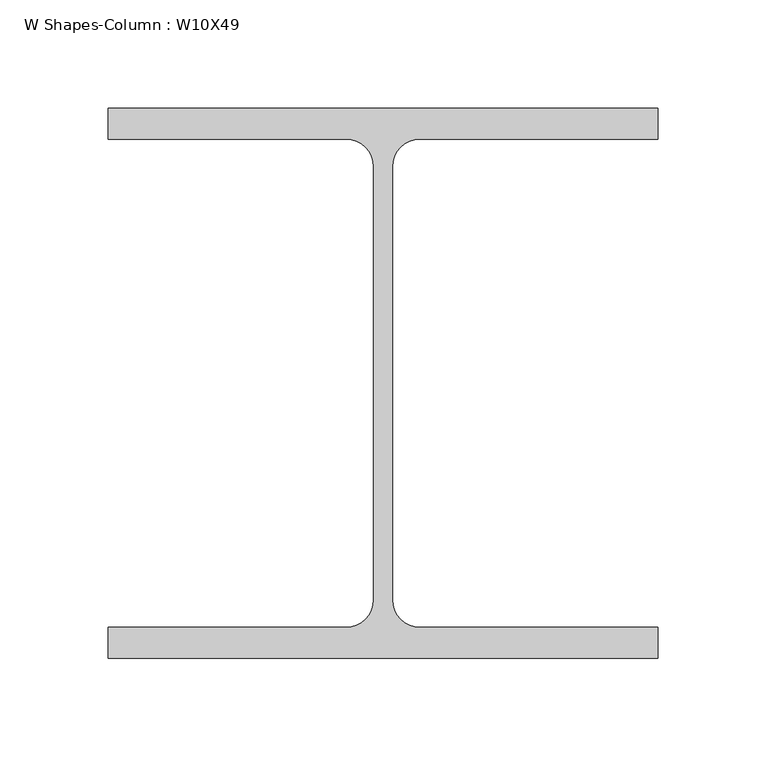
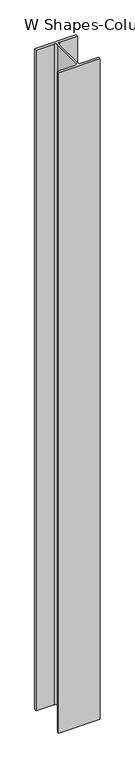
"""IFC4 building model written with IfcOpenShell, lengths in millimetres: column geometry, W Shapes-Column : W10X49."""

from ifc_helpers import new_model, si_unit, point, frame_2d, origin, origin_with_axes, place, context, project, spatial, polyline, circle_curve, trimmed, segment, composite_curve, outline, extrude, source, transform, mapped, element, save


def w_shapes_column_w10x49_053c6d64(model_context):
    return source(origin(), model_context, "Body", "SweptSolid", [
        extrude(outline(composite_curve([segment(polyline([(127.0, 127.0), (127.0, 112.776), (17.018, 112.776)]), True, "CONTINUOUS"), segment(trimmed(circle_curve(frame_2d((17.018, 100.076)), 12.7), [point((17.018, 112.776))], [point((4.318, 100.076))], True, "CARTESIAN"), True, "CONTINUOUS"), segment(polyline([(4.318, 100.076), (4.318, -100.076)]), True, "CONTINUOUS"), segment(trimmed(circle_curve(frame_2d((17.018, -100.076)), 12.7), [point((4.318, -100.076))], [point((17.018, -112.776))], True, "CARTESIAN"), True, "CONTINUOUS"), segment(polyline([(17.018, -112.776), (127.0, -112.776), (127.0, -127.0), (-127.0, -127.0), (-127.0, -112.776), (-17.018, -112.776)]), True, "CONTINUOUS"), segment(trimmed(circle_curve(frame_2d((-17.018, -100.076)), 12.7), [point((-17.018, -112.776))], [point((-4.318, -100.076))], True, "CARTESIAN"), True, "CONTINUOUS"), segment(polyline([(-4.318, -100.076), (-4.318, 100.076)]), True, "CONTINUOUS"), segment(trimmed(circle_curve(frame_2d((-17.018, 100.076)), 12.7), [point((-4.318, 100.076))], [point((-17.018, 112.776))], True, "CARTESIAN"), True, "CONTINUOUS"), segment(polyline([(-17.018, 112.776), (-127.0, 112.776), (-127.0, 127.0), (127.0, 127.0)]), True, "CONTINUOUS")], self_intersect=False)), origin_with_axes(), (0.0, 0.0, 1.0), 4267.0),
    ])


if __name__ == "__main__":
    model = new_model("IFC4")
    model_context = context("Model", 3, world=origin())
    ifc_project = project(units=[si_unit("LENGTHUNIT", "METRE", prefix="MILLI")], contexts=[model_context])
    site = spatial("IfcSite", under=ifc_project)
    building = spatial("IfcBuilding", under=site)
    placement = place(None, origin())
    w_shapes_column_w10x49_shape = w_shapes_column_w10x49_053c6d64(model_context)
    element("IfcColumn", 1, ObjectType="W Shapes-Column : W10X49", at=placement, inside=building, context=model_context, shape_type="MappedRepresentation", body=[
        mapped(w_shapes_column_w10x49_shape, transform((0.0, 0.0, 0.0), x_axis=(1.0, 0.0, 0.0), y_axis=(0.0, 1.0, 0.0), z_axis=(0.0, 0.0, 1.0))),
    ])
    save(model, "model.ifc")

# Revit data of these elements
# Type "W Shapes-Column : W10X49"
#   Section Name Key = "W10X49"
#   Width = 10.000"
#   Web Thickness = 0.340"
#   Web Fillet = 0.500"
#   Warping Constant = 2070.00 in⁶
#   Torsional Moment of Inertia = 1.39 in⁴
#   Section Area = 14.40 in²
#   Plastic Modulus weak axis = 28.30 in³
#   Plastic Modulus strong axis = 60.40 in³
#   Perimeter = 4.875 ft²/ft
#   Nominal Weight = 49.00 lbf/ft
#   Moment of Inertia weak axis = 93.40 in⁴
#   Moment of Inertia strong axis = 272.00 in⁴
#   Height = 10.000"
#   Flange Thickness = 0.560"
#   Elastic Modulus weak axis = 18.70 in³
#   Elastic Modulus strong axis = 54.60 in³
#   Clear Web Height = 0' - 7 1/2"
#   Centroid Vertical = 5.000"
#   Centroid Horizontal = 5.000"
#   Bolt Spacing = 0' - 5 1/2"
#   Structural Material [instance default] = Steel ASTM A992
#   Principal Axes Angle = 0
# Element 1 (IfcColumn, "W Shapes-Column : W10X49")
#   Materials on its faces: "Steel ASTM A992"
# Materials
#   "Steel ASTM A992": class "Metal", colour RGB 199 199 199, transparency 0, Description = "Structural steel 50ksi", Cost = 0
